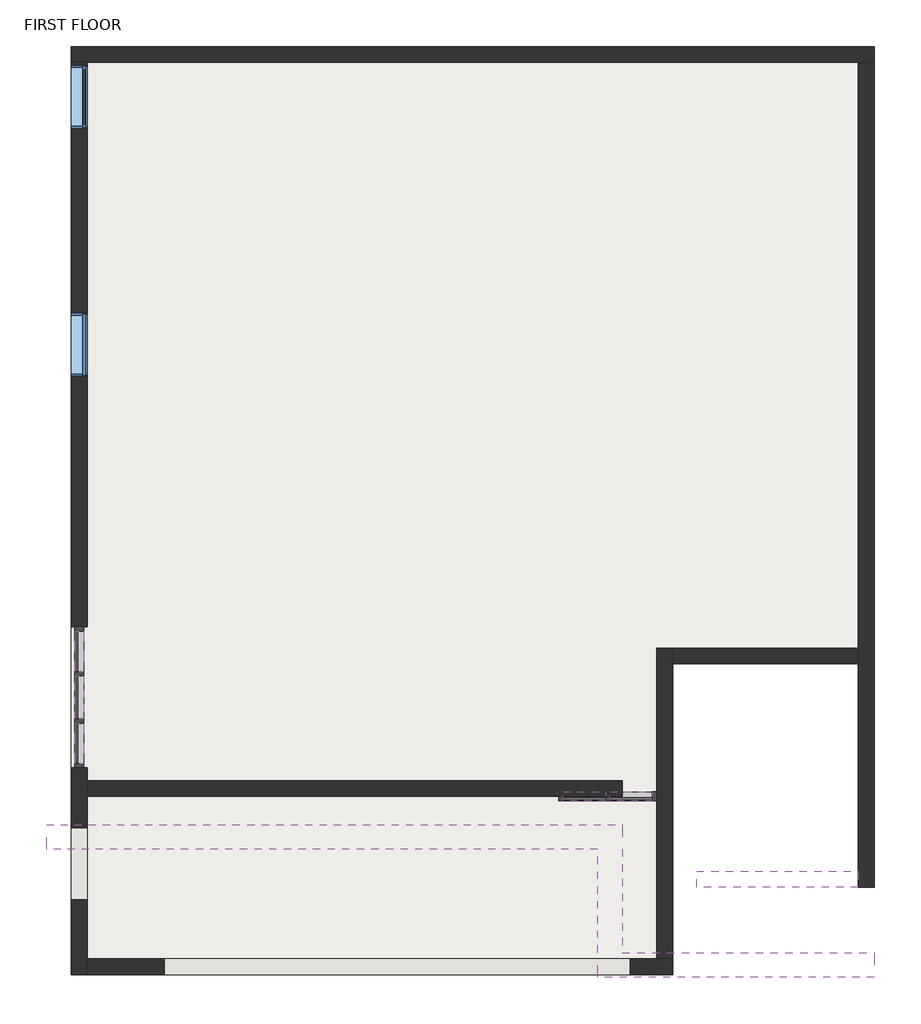
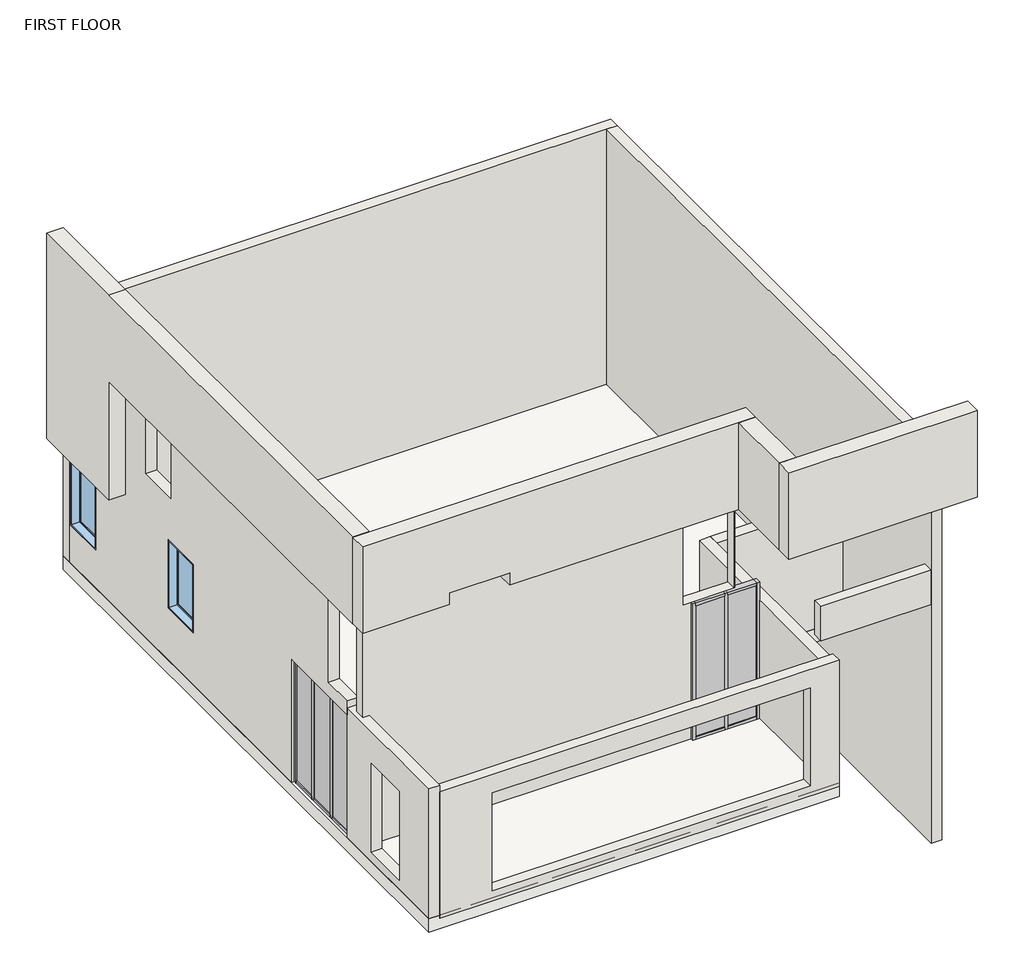
# One storey: 17 members, 10 walls, 5 plates, 2 windows, 1 slab.
"""IFC4 building model written with IfcOpenShell, lengths in millimetres."""

from ifc_helpers import new_model, si_unit, frame, origin, place, context, project, spatial, polyline, outline, extrude, faceted_brep, transform, mapped, element, save
from components import member_a78380a5, member_818e9b4f, member_923d5781, member_94110371, member_3f395ae9, member_47bfaf8a, member_eaba9652, system_panel_glazed_aba10d55, system_panel_glazed_f1f14fe1, system_panel_glazed_7c349084, walls_3_walls_3_ce3253ed, window_cd393ee1

model = new_model("IFC4")

# Units and contexts
model_context = context("Model", 3, world=origin())
ifc_project = project(units=[si_unit("LENGTHUNIT", "METRE", prefix="MILLI")], contexts=[model_context])

# Site, building, storey
site = spatial("IfcSite", under=ifc_project)
building = spatial("IfcBuilding", under=site)
storey = spatial("IfcBuildingStorey", under=building, Name="FIRST FLOOR", Elevation=3048.0)

# Members
placement = place(None, origin())
member_shape = member_a78380a5(model_context)
element("IfcMember", 1, ObjectType="Rectangular Mullion : 2.5\" x 5\" rectangular", at=placement, inside=storey, context=model_context, shape_type="MappedRepresentation", body=[
    mapped(member_shape, transform((-7703.3081251, 4742.1873118, 3048.0), x_axis=(0.0, 1.0, 0.0), y_axis=(1.0, 0.0, 0.0), z_axis=(0.0, 0.0, -1.0))),
])
element("IfcMember", 2, ObjectType="Rectangular Mullion : 2.5\" x 5\" rectangular", at=placement, inside=storey, context=model_context, shape_type="MappedRepresentation", body=[
    mapped(member_shape, transform((-7703.3081251, 2710.1873118, 5791.2), x_axis=(0.0, -1.0, 0.0), y_axis=(1.0, 0.0, 0.0), z_axis=(0.0, 0.0, 1.0))),
])
member_2_shape = member_818e9b4f(model_context)
element("IfcMember", 3, ObjectType="Rectangular Mullion : 2.5\" x 5\" rectangular", at=placement, inside=storey, context=model_context, shape_type="MappedRepresentation", body=[
    mapped(member_2_shape, transform((-7703.3081251, 4678.6873118, 5791.2), x_axis=(0.0, 0.0, 1.0), y_axis=(1.0, 0.0, 0.0), z_axis=(0.0, 1.0, 0.0))),
])
element("IfcMember", 4, ObjectType="Rectangular Mullion : 2.5\" x 5\" rectangular", at=placement, inside=storey, context=model_context, shape_type="MappedRepresentation", body=[
    mapped(member_2_shape, transform((-7703.3081251, 3355.7706451, 5791.2), x_axis=(0.0, 0.0, 1.0), y_axis=(1.0, 0.0, 0.0), z_axis=(0.0, 1.0, 0.0))),
])
element("IfcMember", 5, ObjectType="Rectangular Mullion : 2.5\" x 5\" rectangular", at=placement, inside=storey, context=model_context, shape_type="MappedRepresentation", body=[
    mapped(member_2_shape, transform((-7703.3081251, 2773.6873118, 3048.0), x_axis=(0.0, 0.0, -1.0), y_axis=(1.0, 0.0, 0.0), z_axis=(0.0, -1.0, 0.0))),
])
element("IfcMember", 6, ObjectType="Rectangular Mullion : 2.5\" x 5\" rectangular", at=placement, inside=storey, context=model_context, shape_type="MappedRepresentation", body=[
    mapped(member_2_shape, transform((-7703.3081251, 4096.6039785, 3048.0), x_axis=(0.0, 0.0, -1.0), y_axis=(1.0, 0.0, 0.0), z_axis=(0.0, -1.0, 0.0))),
])
member_3_shape = member_923d5781(model_context)
element("IfcMember", 7, ObjectType="Rectangular Mullion : 2.5\" x 5\" rectangular", at=placement, inside=storey, context=model_context, shape_type="MappedRepresentation", body=[
    mapped(member_3_shape, transform((-7703.3081251, 4064.8539785, 3048.0), x_axis=(0.0, 1.0, 0.0), y_axis=(1.0, 0.0, 0.0), z_axis=(0.0, 0.0, -1.0))),
])
element("IfcMember", 8, ObjectType="Rectangular Mullion : 2.5\" x 5\" rectangular", at=placement, inside=storey, context=model_context, shape_type="MappedRepresentation", body=[
    mapped(member_3_shape, transform((-7703.3081251, 3387.5206451, 3048.0), x_axis=(0.0, 1.0, 0.0), y_axis=(1.0, 0.0, 0.0), z_axis=(0.0, 0.0, -1.0))),
])
member_4_shape = member_94110371(model_context)
element("IfcMember", 9, ObjectType="Rectangular Mullion : 2.5\" x 5\" rectangular", at=placement, inside=storey, context=model_context, shape_type="MappedRepresentation", body=[
    mapped(member_4_shape, transform((-7703.3081251, 4033.1039785, 5791.2), x_axis=(0.0, 0.0, 1.0), y_axis=(1.0, 0.0, 0.0), z_axis=(0.0, 1.0, 0.0))),
])
element("IfcMember", 10, ObjectType="Rectangular Mullion : 2.5\" x 5\" rectangular", at=placement, inside=storey, context=model_context, shape_type="MappedRepresentation", body=[
    mapped(member_4_shape, transform((-7703.3081251, 3419.2706451, 3048.0), x_axis=(0.0, 0.0, -1.0), y_axis=(1.0, 0.0, 0.0), z_axis=(0.0, -1.0, 0.0))),
])
member_5_shape = member_3f395ae9(model_context)
element("IfcMember", 11, ObjectType="Rectangular Mullion : 2.5\" x 5\" rectangular", at=placement, inside=storey, context=model_context, shape_type="MappedRepresentation", body=[
    mapped(member_5_shape, transform((-807.1207252, 2301.5467494, 3048.0), x_axis=(-1.0, 0.0, 0.0), y_axis=(0.0, 1.0, 0.0), z_axis=(0.0, 0.0, -1.0))),
])
element("IfcMember", 12, ObjectType="Rectangular Mullion : 2.5\" x 5\" rectangular", at=placement, inside=storey, context=model_context, shape_type="MappedRepresentation", body=[
    mapped(member_5_shape, transform((602.5792748, 2301.5467494, 6096.0), x_axis=(1.0, 0.0, 0.0), y_axis=(0.0, 1.0, 0.0), z_axis=(0.0, 0.0, 1.0))),
])
member_6_shape = member_47bfaf8a(model_context)
element("IfcMember", 13, ObjectType="Rectangular Mullion : 2.5\" x 5\" rectangular", at=placement, inside=storey, context=model_context, shape_type="MappedRepresentation", body=[
    mapped(member_6_shape, transform((-743.6207252, 2301.5467494, 6096.0), x_axis=(0.0, 0.0, 1.0), y_axis=(0.0, 1.0, 0.0), z_axis=(-1.0, 0.0, 0.0))),
])
element("IfcMember", 14, ObjectType="Rectangular Mullion : 2.5\" x 5\" rectangular", at=placement, inside=storey, context=model_context, shape_type="MappedRepresentation", body=[
    mapped(member_6_shape, transform((-70.5207252, 2301.5467494, 6096.0), x_axis=(0.0, 0.0, 1.0), y_axis=(0.0, 1.0, 0.0), z_axis=(-1.0, 0.0, 0.0))),
])
element("IfcMember", 15, ObjectType="Rectangular Mullion : 2.5\" x 5\" rectangular", at=placement, inside=storey, context=model_context, shape_type="MappedRepresentation", body=[
    mapped(member_6_shape, transform((539.0792748, 2301.5467494, 3048.0), x_axis=(0.0, 0.0, -1.0), y_axis=(0.0, 1.0, 0.0), z_axis=(1.0, 0.0, 0.0))),
])
element("IfcMember", 16, ObjectType="Rectangular Mullion : 2.5\" x 5\" rectangular", at=placement, inside=storey, context=model_context, shape_type="MappedRepresentation", body=[
    mapped(member_6_shape, transform((-134.0207252, 2301.5467494, 3048.0), x_axis=(0.0, 0.0, -1.0), y_axis=(0.0, 1.0, 0.0), z_axis=(1.0, 0.0, 0.0))),
])
member_7_shape = member_eaba9652(model_context)
element("IfcMember", 17, ObjectType="Rectangular Mullion : 2.5\" x 5\" rectangular", at=placement, inside=storey, context=model_context, shape_type="MappedRepresentation", body=[
    mapped(member_7_shape, transform((-102.2707252, 2301.5467494, 3048.0), x_axis=(-1.0, 0.0, 0.0), y_axis=(0.0, 1.0, 0.0), z_axis=(0.0, 0.0, -1.0))),
])

# Plates
system_panel_glazed_shape = system_panel_glazed_aba10d55(model_context)
element("IfcPlate", 18, ObjectType="System Panel : Glazed", at=placement, inside=storey, context=model_context, shape_type="MappedRepresentation", body=[
    mapped(system_panel_glazed_shape, transform((-7703.3081251, 3064.7289785, 3111.5), x_axis=(0.0, 1.0, 0.0), y_axis=(-1.0, 0.0, 0.0), z_axis=(0.0, 0.0, 1.0))),
])
element("IfcPlate", 19, ObjectType="System Panel : Glazed", at=placement, inside=storey, context=model_context, shape_type="MappedRepresentation", body=[
    mapped(system_panel_glazed_shape, transform((-7703.3081251, 4387.6456451, 3111.5), x_axis=(0.0, 1.0, 0.0), y_axis=(-1.0, 0.0, 0.0), z_axis=(0.0, 0.0, 1.0))),
])
system_panel_glazed_2_shape = system_panel_glazed_f1f14fe1(model_context)
element("IfcPlate", 20, ObjectType="System Panel : Glazed", at=placement, inside=storey, context=model_context, shape_type="MappedRepresentation", body=[
    mapped(system_panel_glazed_2_shape, transform((-7703.3081251, 3726.1873118, 3111.5), x_axis=(0.0, 1.0, 0.0), y_axis=(-1.0, 0.0, 0.0), z_axis=(0.0, 0.0, 1.0))),
])
system_panel_glazed_3_shape = system_panel_glazed_7c349084(model_context)
element("IfcPlate", 21, ObjectType="System Panel : Glazed", at=placement, inside=storey, context=model_context, shape_type="MappedRepresentation", body=[
    mapped(system_panel_glazed_3_shape, transform((234.2792748, 2301.5467494, 3111.5), x_axis=(-1.0, 0.0, 0.0), y_axis=(0.0, -1.0, 0.0), z_axis=(0.0, 0.0, 1.0))),
])
element("IfcPlate", 22, ObjectType="System Panel : Glazed", at=placement, inside=storey, context=model_context, shape_type="MappedRepresentation", body=[
    mapped(system_panel_glazed_3_shape, transform((-438.8207252, 2301.5467494, 3111.5), x_axis=(-1.0, 0.0, 0.0), y_axis=(0.0, -1.0, 0.0), z_axis=(0.0, 0.0, 1.0))),
])

# Slab
element("IfcSlab", 23, ObjectType="Generic - 12\"", at=placement, inside=storey, context=model_context, shape_type="SweptSolid", body=[
    extrude(outline(polyline([(3726.6918749, 13083.8953049), (3726.6918749, 4206.5953049), (831.1792748, 4206.5953049), (831.1792748, -263.8046951), (-7817.6081251, -263.8046951), (-7817.6081251, 13083.8953049), (3726.6918749, 13083.8953049)])), frame((0.0, 0.0, 2743.2), z_axis=(0.0, 0.0, 1.0), x_axis=(1.0, 0.0, 0.0)), (0.0, 0.0, 1.0), 304.8),
])

# Walls
element("IfcWall", 24, ObjectType="9\"", at=placement, inside=storey, context=model_context, shape_type="Brep", body=[
    faceted_brep([(-7817.6081251, 12855.2953049, 3048.0), (-7589.0081251, 12855.2953049, 3048.0), (-6636.5081251, 12855.2953049, 3048.0), (3498.0918749, 12855.2953049, 3048.0), (3726.6918749, 12855.2953049, 3048.0), (3726.6918749, 12855.2953049, 8737.6), (3498.0918749, 12855.2953049, 8737.6), (-7817.6081251, 12855.2953049, 8737.6), (-7817.6081251, 12855.2953049, 8432.8), (-7817.6081251, 13083.8953049, 3048.0), (-7817.6081251, 13083.8953049, 8737.6), (3726.6918749, 13083.8953049, 8737.6), (3726.6918749, 13083.8953049, 3048.0), (3498.0918749, 13083.8953049, 3048.0), (-6636.5081251, 13083.8953049, 3048.0)], [[[0, 1, 2, 3, 4, 5, 6, 7, 8]], [[9, 10, 11, 12, 13, 14]], [[4, 3, 2, 1, 0, 9, 14, 13, 12]], [[7, 6, 5, 11, 10]], [[5, 4, 12, 11]], [[0, 8, 7, 10, 9]]]),
])
element("IfcWall", 25, ObjectType="9\"", at=placement, inside=storey, context=model_context, shape_type="Brep", body=[
    faceted_brep([(3498.0918749, 13083.8953049, 0.0), (3498.0918749, 12855.2953049, 0.0), (3498.0918749, 993.4953049, 0.0), (3498.0918749, 993.4953049, 5334.0), (3498.0918749, 993.4953049, 6096.0), (3498.0918749, 993.4953049, 8737.6), (3498.0918749, 12855.2953049, 8737.6), (3498.0918749, 12855.2953049, 3048.0), (3498.0918749, 13083.8953049, 3048.0), (3726.6918749, 13083.8953049, 0.0), (3726.6918749, 13083.8953049, 3048.0), (3726.6918749, 12855.2953049, 3048.0), (3726.6918749, 12855.2953049, 8737.6), (3726.6918749, 993.4953049, 8737.6), (3726.6918749, 993.4953049, 0.0)], [[[0, 1, 2, 3, 4, 5, 6, 7, 8]], [[9, 10, 11, 12, 13, 14]], [[2, 1, 0, 9, 14]], [[6, 5, 13, 12]], [[5, 4, 3, 2, 14, 13]], [[7, 11, 10, 8]], [[0, 8, 10, 9]], [[7, 6, 12, 11]]]),
])
element("IfcWall", 26, ObjectType="9\"", at=placement, inside=storey, context=model_context, shape_type="Brep", body=[
    faceted_brep([(-7589.0081251, -263.8046951, 3048.0), (-7589.0081251, 2710.1873118, 3048.0), (-7589.0081251, 2710.1873118, 5791.2), (-7589.0081251, 2710.1873118, 5943.6), (-7589.0081251, -263.8046951, 5943.6), (-7589.0081251, -263.8046951, 5791.2), (-7589.0081251, 1847.3885721, 5232.4), (-7589.0081251, 1847.3885721, 3251.2), (-7589.0081251, 815.6953049, 3251.2), (-7589.0081251, 815.6953049, 5232.4), (-7817.6081251, -263.8046951, 3048.0), (-7817.6081251, -263.8046951, 5943.6), (-7817.6081251, 2710.1873118, 5943.6), (-7817.6081251, 2710.1873118, 5791.2), (-7817.6081251, 2710.1873118, 3048.0), (-7817.6081251, 1847.3885721, 5232.4), (-7817.6081251, 815.6953049, 5232.4), (-7817.6081251, 815.6953049, 3251.2), (-7817.6081251, 1847.3885721, 3251.2)], [[[0, 1, 2, 3, 4, 5], [6, 7, 8, 9]], [[10, 11, 12, 13, 14], [15, 16, 17, 18]], [[1, 0, 10, 14]], [[3, 2, 1, 14, 13, 12]], [[4, 3, 12, 11]], [[7, 6, 15, 18]], [[8, 7, 18, 17]], [[9, 8, 17, 16]], [[6, 9, 16, 15]], [[0, 5, 4, 11, 10]]]),
])
element("IfcWall", 27, ObjectType="9\"", at=placement, inside=storey, context=model_context, shape_type="SweptSolid", body=[
    extrude(outline(polyline([(1173.9918749, 1222.0953049), (3498.0918749, 1222.0953049), (3498.0918749, 993.4953049), (1173.9918749, 993.4953049), (1173.9918749, 1222.0953049)])), frame((0.0, 0.0, 5334.0), z_axis=(0.0, 0.0, 1.0), x_axis=(1.0, 0.0, 0.0)), (0.0, 0.0, 1.0), 762.0),
])
element("IfcWall", 28, ObjectType="9\"", at=placement, inside=storey, context=model_context, shape_type="Brep", body=[
    faceted_brep([(-7589.0081251, -263.8046951, 2971.8), (831.1792748, -263.8046951, 2971.8), (831.1792748, -263.8046951, 5791.2), (-7589.0081251, -263.8046951, 5791.2), (-7589.0081251, -263.8046951, 3048.0), (221.4918749, -263.8046951, 5384.8), (221.4918749, -263.8046951, 3200.4), (-6484.1081251, -263.8046951, 3200.4), (-6484.1081251, -263.8046951, 5384.8), (-7589.0081251, -35.2046951, 2971.8), (-7589.0081251, -35.2046951, 5791.2), (831.1792748, -35.2046951, 5791.2), (831.1792748, -35.2046951, 5689.6), (831.1792748, -35.2046951, 3048.0), (831.1792748, -35.2046951, 2971.8), (221.4918749, -35.2046951, 5384.8), (-6484.1081251, -35.2046951, 5384.8), (-6484.1081251, -35.2046951, 3200.4), (221.4918749, -35.2046951, 3200.4)], [[[0, 1, 2, 3, 4], [5, 6, 7, 8]], [[9, 10, 11, 12, 13, 14], [15, 16, 17, 18]], [[0, 4, 3, 10, 9]], [[2, 1, 14, 13, 12, 11]], [[1, 0, 9, 14]], [[3, 2, 11, 10]], [[6, 5, 15, 18]], [[7, 6, 18, 17]], [[8, 7, 17, 16]], [[5, 8, 16, 15]]]),
])
element("IfcWall", 29, ObjectType="9\"", at=placement, inside=storey, context=model_context, shape_type="Brep", body=[
    faceted_brep([(831.1792748, -35.2046951, 3048.0), (831.1792748, 4206.5953049, 3048.0), (831.1792748, 4435.1953049, 3048.0), (831.1792748, 4435.1953049, 5689.6), (831.1792748, 4206.5953049, 5689.6), (831.1792748, -35.2046951, 5689.6), (602.5792748, -35.2046951, 3048.0), (602.5792748, -35.2046951, 5689.6), (602.5792748, 4435.1953049, 5689.6), (602.5792748, 4435.1953049, 3048.0)], [[[0, 1, 2, 3, 4, 5]], [[6, 7, 8, 9]], [[2, 1, 0, 6, 9]], [[5, 4, 3, 8, 7]], [[0, 5, 7, 6]], [[3, 2, 9, 8]]]),
])
element("IfcWall", 30, ObjectType="9\"", at=placement, inside=storey, context=model_context, shape_type="SweptSolid", body=[
    extrude(outline(polyline([(3498.0918749, 4206.5953049), (831.1792748, 4206.5953049), (831.1792748, 4435.1953049), (3498.0918749, 4435.1953049), (3498.0918749, 4206.5953049)])), frame((0.0, 0.0, 3048.0), z_axis=(0.0, 0.0, 1.0), x_axis=(1.0, 0.0, 0.0)), (0.0, 0.0, 1.0), 2641.6),
])
element("IfcWall", 31, ObjectType="9\"", at=placement, inside=storey, context=model_context, shape_type="SweptSolid", body=[
    extrude(outline(polyline([(3048.0, -7728.7081251), (3048.0, 107.2792748), (8532.3627235, 107.2792748), (8532.3627235, -7728.7081251), (3048.0, -7728.7081251)]), holes=[polyline([(6096.0, -972.2207252), (8432.8, -972.2207252), (8432.8, 94.5792748), (6096.0, 94.5792748), (6096.0, -972.2207252)])]), frame((0.0, 2301.5467494, 0.0), z_axis=(0.0, 1.0, 0.0), x_axis=(0.0, 0.0, 1.0)), (0.0, 0.0, 1.0), 228.6),
])
element("IfcWall", 32, ObjectType="9\"", at=placement, inside=storey, context=model_context, shape_type="Brep", body=[
    faceted_brep([(-7589.0081251, 12855.2953049, 3048.0), (-7589.0081251, 12855.2953049, 8432.8), (-7589.0081251, 3404.9615229, 8432.8), (-7589.0081251, 3404.9615229, 6096.0), (-7589.0081251, 2710.1873118, 6096.0), (-7589.0081251, 2710.1873118, 5943.6), (-7589.0081251, 2710.1873118, 5791.2), (-7589.0081251, 4742.1873118, 5791.2), (-7589.0081251, 4742.1873118, 3048.0), (-7589.0081251, 8340.4453049, 4206.4403624), (-7589.0081251, 8340.4453049, 5730.4403624), (-7589.0081251, 9254.8453049, 5730.4403624), (-7589.0081251, 9254.8453049, 4206.4403624), (-7589.0081251, 11902.7953049, 3889.390202), (-7589.0081251, 11902.7953049, 5413.390202), (-7589.0081251, 12817.1953049, 5413.390202), (-7589.0081251, 12817.1953049, 3889.390202), (-7589.0081251, 9159.5953049, 6705.6), (-7589.0081251, 9159.5953049, 8229.6), (-7589.0081251, 10073.9953049, 8229.6), (-7589.0081251, 10073.9953049, 6705.6), (-7817.6081251, 12855.2953049, 8432.8), (-7817.6081251, 12855.2953049, 3048.0), (-7817.6081251, 4742.1873118, 3048.0), (-7817.6081251, 4742.1873118, 5791.2), (-7817.6081251, 2710.1873118, 5791.2), (-7817.6081251, 2710.1873118, 5943.6), (-7817.6081251, 2710.1873118, 6096.0), (-7817.6081251, 3404.9615229, 6096.0), (-7817.6081251, 3404.9615229, 8432.8), (-7817.6081251, 8340.4453049, 5730.4403624), (-7817.6081251, 8340.4453049, 4206.4403624), (-7817.6081251, 9254.8453049, 4206.4403624), (-7817.6081251, 9254.8453049, 5730.4403624), (-7817.6081251, 11902.7953049, 5413.390202), (-7817.6081251, 11902.7953049, 3889.390202), (-7817.6081251, 12817.1953049, 3889.390202), (-7817.6081251, 12817.1953049, 5413.390202), (-7817.6081251, 9159.5953049, 8229.6), (-7817.6081251, 9159.5953049, 6705.6), (-7817.6081251, 10073.9953049, 6705.6), (-7817.6081251, 10073.9953049, 8229.6)], [[[0, 1, 2, 3, 4, 5, 6, 7, 8], [9, 10, 11, 12], [13, 14, 15, 16], [17, 18, 19, 20]], [[21, 22, 23, 24, 25, 26, 27, 28, 29], [30, 31, 32, 33], [34, 35, 36, 37], [38, 39, 40, 41]], [[1, 21, 29, 2]], [[22, 0, 8, 23]], [[25, 6, 5, 4, 27, 26]], [[1, 0, 22, 21]], [[24, 7, 6, 25]], [[7, 24, 23, 8]], [[28, 3, 2, 29]], [[3, 28, 27, 4]], [[31, 30, 10, 9]], [[32, 31, 9, 12]], [[33, 32, 12, 11]], [[30, 33, 11, 10]], [[35, 34, 14, 13]], [[36, 35, 13, 16]], [[37, 36, 16, 15]], [[34, 37, 15, 14]], [[38, 18, 17, 39]], [[39, 17, 20, 40]], [[40, 20, 19, 41]], [[18, 38, 41, 19]]]),
])
walls_3_walls_3_shape = walls_3_walls_3_ce3253ed(model_context)
element("IfcWall", 33, ObjectType="Walls 3 : Walls 3", at=placement, inside=storey, context=model_context, shape_type="MappedRepresentation", body=[
    mapped(walls_3_walls_3_shape, transform((0.0, 0.0, 0.0), x_axis=(1.0, 0.0, 0.0), y_axis=(0.0, 1.0, 0.0), z_axis=(0.0, 0.0, 1.0))),
])

# Windows
window_shape = window_cd393ee1(model_context)
element("IfcWindow", 34, ObjectType="Fixed : 36\" x 48\"", at=placement, inside=storey, context=model_context, shape_type="MappedRepresentation", body=[
    mapped(window_shape, transform((-7703.3081251, 8759.5453049, 3292.0403624), x_axis=(0.0, -1.0, 0.0), y_axis=(1.0, 0.0, 0.0), z_axis=(0.0, 0.0, 1.0))),
])
element("IfcWindow", 35, ObjectType="Fixed : 36\" x 48\"", at=placement, inside=storey, context=model_context, shape_type="MappedRepresentation", body=[
    mapped(window_shape, transform((-7703.3081251, 12321.8953049, 2974.990202), x_axis=(0.0, -1.0, 0.0), y_axis=(1.0, 0.0, 0.0), z_axis=(0.0, 0.0, 1.0))),
])

save(model, "model.ifc")

# Revit data of these elements
# Type "Rectangular Mullion : 2.5\" x 5\" rectangular"
#   built-in parameter 1007304 = 0.416667 (stored number, unit not read)
#   built-in parameter 1007301 = 0.104167 (stored number, unit not read)
#   built-in parameter 1007300 = 0.104167 (stored number, unit not read)
# Type "System Panel : Glazed"
#   Construction Type Id = "GSP4R"
#   Analytic Construction = "1/8 in Pilkington single glazing"
#   Visual Light Transmittance = 0.9
#   Solar Heat Gain Coefficient = 0.86
#   Heat Transfer Coefficient (U) = 1.18115 BTU/(h·ft²·°F)
#   Define Thermal Properties by = 1
# Type "Generic - 12\""
#   Assembly Code = "B1010"
#   Function = 0
#   Layers, outside or top first: 1' - 0" no material (function 1)
# Type "9\""
#   Assembly Code = "B2010"
#   Layers, outside or top first: 0' - 9" "1 wall" (function 1)
# Type "Fixed : 36\" x 48\""
#   Type Mark = "1"
#   Construction Type Id = "GSP4R"
#   Assembly Code = "B2020100"
#   Analytic Construction = "1/8 in Pilkington single glazing"
#   Visual Light Transmittance = 0.9
#   Solar Heat Gain Coefficient = 0.78
#   Heat Transfer Coefficient (U) = 0.6496 BTU/(h·ft²·°F)
#   Height = 5' - 0"
#   Default Sill Height = 3' - 0"
#   Width = 3' - 0"
#   Window Inset = 0' - 0 3/4"
#   Define Thermal Properties by = 1
#   Define Thermal Properties by = 1
#   Glass Pane Material = Glass
#   Sash Material = Sash
#   Wall Closure = (empty or 0)
# Elements 1, 2, 3, 4, 5, 6, 7, 8, 9, 10, 11, 12, 13, 14, 15, 16, 17 (IfcMember, "Rectangular Mullion : 2.5\" x 5\" rectangular")
#   Phase Created = New Construction
#   Materials on its faces: "Aluminum"
# Elements 18, 19, 20, 21, 22 (IfcPlate, "System Panel : Glazed")
#   Phase Created = New Construction
#   Materials on its faces: "Glass"
# Element 23 (IfcSlab, "Generic - 12\"")
#   Height Offset From Level = 0' - 0"
#   Phase Created = New Construction
#   Materials on its faces: "Default Floor", "Acoustic Ceiling Tile 24 x 24", "1 white"
# Element 24 (IfcWall, "9\"")
#   Top Offset = 0' - 0"
#   Base Offset = 0' - 0"
#   Unconnected Height = 18' - 8"
#   wall height = 18' - 8"
#   Phase Created = New Construction
#   Base Constraint = FIRST FLOOR
#   Materials on its faces: "1 wall"
# Element 25 (IfcWall, "9\"")
#   built-in parameter 1001111 = -10' - 0"
#   Top Offset = 0' - 0"
#   Base Offset = -10' - 0"
#   Unconnected Height = 28' - 8"
#   wall height = 28' - 8"
#   Phase Created = New Construction
#   Base Constraint = FIRST FLOOR
#   Materials on its faces: "1 wall"
# Elements 26, 32 (IfcWall, "9\"")
#   Top Offset = 0' - 0"
#   Base Offset = 0' - 0"
#   Unconnected Height = 17' - 8"
#   wall height = 17' - 8"
#   Phase Created = New Construction
#   Base Constraint = FIRST FLOOR
#   Materials on its faces: "1 wall"
# Element 27 (IfcWall, "9\"")
#   built-in parameter 1001111 = 7' - 6"
#   Top Offset = 0' - 0"
#   Base Offset = 7' - 6"
#   Unconnected Height = 2' - 6"
#   wall height = 2' - 6"
#   Phase Created = New Construction
#   Base Constraint = FIRST FLOOR
#   Materials on its faces: "1 wall"
# Element 28 (IfcWall, "9\"")
#   Top Offset = 0' - 0"
#   Base Offset = 0' - 0"
#   Unconnected Height = 9' - 0"
#   wall height = 9' - 0"
#   Phase Created = New Construction
#   Base Constraint = FIRST FLOOR
#   Materials on its faces: "1 wall"
# Elements 29, 30 (IfcWall, "9\"")
#   Top Offset = 0' - 0"
#   Base Offset = 0' - 0"
#   Unconnected Height = 8' - 8"
#   wall height = 8' - 8"
#   Phase Created = New Construction
#   Base Constraint = FIRST FLOOR
#   Materials on its faces: "1 wall"
# Element 31 (IfcWall, "9\"")
#   Top Offset = 0' - 0"
#   Base Offset = 0' - 0"
#   Unconnected Height = 17' - 11.91979"
#   wall height = 17' - 11.91979"
#   Phase Created = New Construction
#   Base Constraint = FIRST FLOOR
#   Materials on its faces: "1 wall"
# Element 33 (IfcWall, "Walls 3 : Walls 3")
#   Phase Created = New Construction
#   Materials on its faces: "1 white", "Default Wall"
# Element 34 (IfcWindow, "Fixed : 36\" x 48\"")
#   Mark = "1"
#   Phase Created = New Construction
#   Materials on its faces: "Sash", "Glass"
# Element 35 (IfcWindow, "Fixed : 36\" x 48\"")
#   Mark = "2"
#   Phase Created = New Construction
#   Materials on its faces: "Sash", "Glass"
# Materials
#   "1 wall": class "Generic", colour RGB 172 157 136, transparency 0, Cost = 0
#   "Glass": class "Glass", colour RGB 0 128 192, transparency 0.75, Description = "Soda Lime Glass", Cost = 0
#   "Sash": class "Wood", colour RGB 224 178 126, transparency 0, Cost = 0
#   "Aluminum": class "Metal", colour RGB 247 247 247, transparency 0, Description = "Aluminum 6061", Cost = 0
#   "Default Floor": colour RGB 128 128 128, transparency 0, Cost = 0
#   "Acoustic Ceiling Tile 24 x 24": class "Generic", colour RGB 232 232 232, transparency 0, Description = "Acoustic Ceiling Tile 24 x 24", Cost = 0
#   "1 white": class "Generic", colour RGB 244 245 241, transparency 0, Cost = 0
#   "Default Wall": colour RGB 128 128 128, transparency 0, Cost = 0
